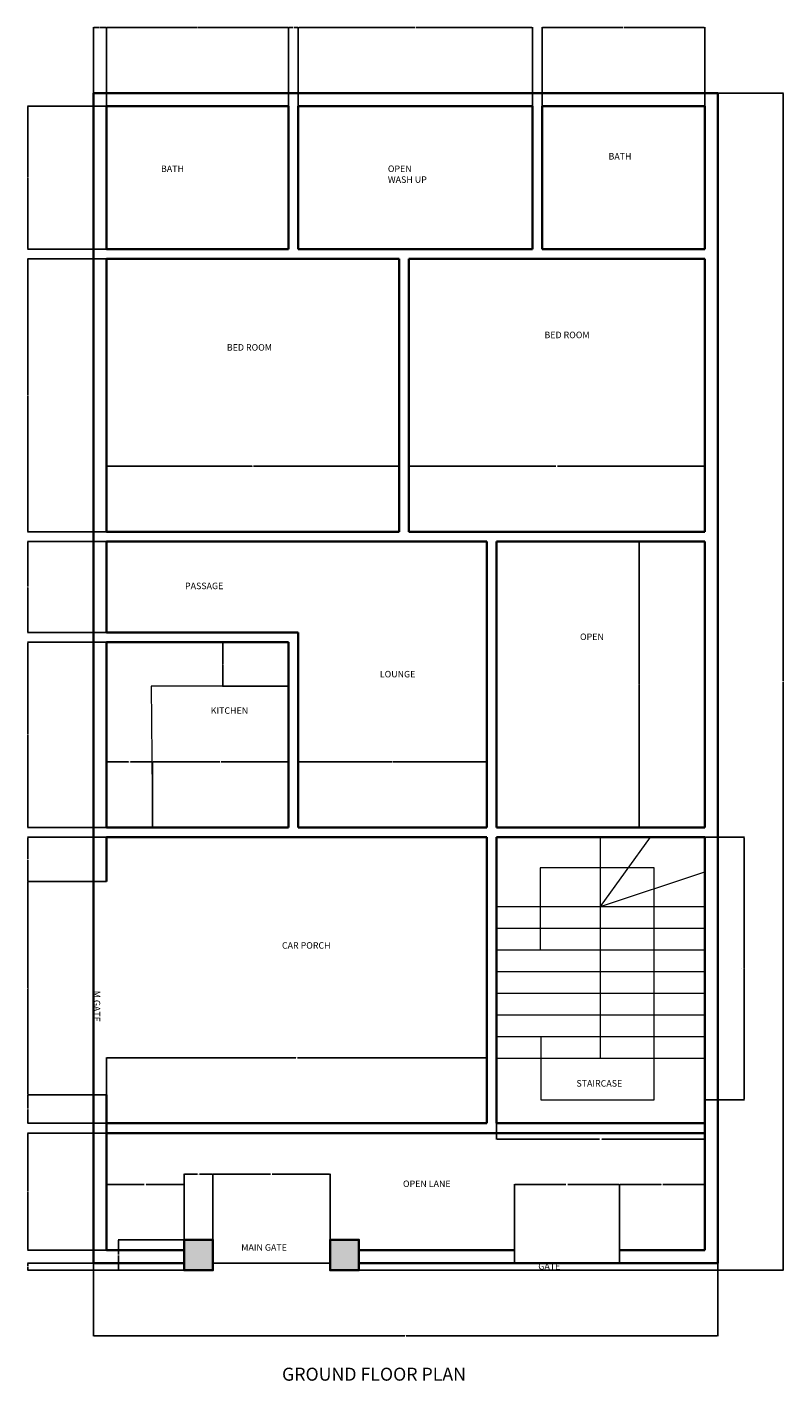
# Model space of a CAD drawing. Units: inches. Extents: x 301 to 1174, y -458 to 167.
# Tile 1 of 4: x 301 to 651, y -458 to 167. Entities that reach past the tile are written whole.
import ezdxf

# ---------------------------------------------------------------- set-up
doc = ezdxf.new("R2010")
doc.units = ezdxf.units.IN
doc.header["$MEASUREMENT"] = 0
for name, color, linetype, lineweight in [('A-ANNO-DIMS', 2, 'Continuous', 18), ('A-ANNO-TEXT', 7, 'Continuous', 25), ('A-AREA-IDEN', 7, 'Continuous', 18), ('A-COLS', 7, 'Continuous', 35), ('A-COLS-PATT', 252, 'Continuous', 13), ('A-DOOR', 3, 'Continuous', 25), ('A-FLOR-FIXT', 8, 'Continuous', 18), ('A-FLOR-STRS', 7, 'Continuous', 18), ('A-WALL', 7, 'Continuous', 35)]:
    doc.layers.add(name, color=color, linetype=linetype, lineweight=lineweight)
doc.styles.get("Standard").update_dxf_attribs({"font": 'arial.ttf'})
doc.dimstyles.get("Standard").update_dxf_attribs({"dimtxt": 0.18, "dimasz": 0.18, "dimexe": 0.18, "dimexo": 0.0625, "dimgap": 0.09, "dimtad": 0, "dimtih": 1, "dimtoh": 1, "dimdec": 4, "dimzin": 0, "dimdsep": 46, "dimtxsty": 'Standard', "dimcen": 0.09, "dimadec": 0, "dimazin": 0, "dimtfac": 1, "dimtdec": 4, "dimtofl": 0, "dimtmove": 0, "dimatfit": 3, "dimfxl": 1, "dimtolj": 1, "dimtzin": 0, "dimarcsym": 0})

# ---------------------------------------------------------------- blocks, each defined once
blk = doc.blocks.new('STAIR-RES-WINDER')
for p, q in [((48, 19.16), (48, 121.12)), ((48, 89.16), (71.07, 121.12)), ((72.66, 107.09), (20.07, 107.09)), ((20.07, 107.09), (20.07, 69.16)), ((72.66, 0), (72.66, 107.09)), ((48, 89.16), (96, 105.1)), ((0, 89.16), (96, 89.16)), ((0, 79.16), (96, 79.16)), ((0, 69.16), (96, 69.16)), ((0, 59.16), (96, 59.16)), ((0, 49.16), (96, 49.16)), ((0, 39.16), (96, 39.16)), ((0, 29.16), (96, 29.16)), ((20.47, 29.16), (20.47, 0)), ((0, 19.16), (96, 19.16)), ((20.47, 0), (72.66, 0))]:
    blk.add_line(p, q)
blk = doc.blocks.new('*D6')
at = {"layer": 'A-ANNO-DIMS', "color": 0, "lineweight": -2, "transparency": 16777216}
for p, q in [((614.09, -206.7), (632.37, -206.7)), ((632.19, -206.88), (632.19, -267.07)), ((632.19, -327.63), (632.19, -267.44)), ((614.09, -327.81), (632.37, -327.81))]:
    blk.add_line(p, q, dxfattribs=at)
at = {"layer": 'A-ANNO-DIMS', "color": 0, "transparency": 16777216}
for points in [[(632.16, -206.88), (632.22, -206.88), (632.19, -206.7)], [(632.16, -327.63), (632.22, -327.63), (632.19, -327.81)]]:
    blk.add_solid(points, dxfattribs=at)
at = {"layer": 'Defpoints', "color": 0, "transparency": 16777216}
for p in [(614.03, -206.7), (632.19, -206.7), (614.03, -327.81)]:
    blk.add_point(p, dxfattribs=at)
at = {"layer": 'A-ANNO-DIMS', "color": 0, "transparency": 16777216, "insert": (632.19, -267.26), "char_height": 0.18, "attachment_point": 5}
blk.add_mtext('\\A1;WINDER STAIR 121 TYP.', dxfattribs=at)
blk = doc.blocks.new('*D7')
at = {"layer": 'A-ANNO-DIMS', "color": 0, "lineweight": -2, "transparency": 16777216}
for p, q in [((518.03, -327.88), (518.03, -346.16)), ((614.03, -327.88), (614.03, -346.16)), ((518.21, -345.98), (565.5, -345.98)), ((613.85, -345.98), (566.55, -345.98))]:
    blk.add_line(p, q, dxfattribs=at)
at = {"layer": 'A-ANNO-DIMS', "color": 0, "transparency": 16777216}
for points in [[(518.21, -345.95), (518.21, -346.01), (518.03, -345.98)], [(613.85, -345.95), (613.85, -346.01), (614.03, -345.98)]]:
    blk.add_solid(points, dxfattribs=at)
at = {"layer": 'Defpoints', "color": 0, "transparency": 16777216}
for p in [(518.03, -327.81), (614.03, -327.81), (614.03, -345.98)]:
    blk.add_point(p, dxfattribs=at)
at = {"layer": 'A-ANNO-DIMS', "color": 0, "transparency": 16777216, "insert": (566.03, -345.98), "char_height": 0.18, "attachment_point": 5}
blk.add_mtext('\\A1;96 TYP.', dxfattribs=at)
blk = doc.blocks.new('*D8')
at = {"layer": 'A-ANNO-DIMS', "color": 0, "lineweight": -2, "transparency": 16777216}
for p, q in [((332.03, -403.26), (332.03, -436.96)), ((620.03, -403.26), (620.03, -436.96)), ((332.21, -436.78), (475.74, -436.78)), ((619.85, -436.78), (476.32, -436.78))]:
    blk.add_line(p, q, dxfattribs=at)
at = {"layer": 'A-ANNO-DIMS', "color": 0, "transparency": 16777216}
for points in [[(332.21, -436.75), (332.21, -436.81), (332.03, -436.78)], [(619.85, -436.75), (619.85, -436.81), (620.03, -436.78)]]:
    blk.add_solid(points, dxfattribs=at)
at = {"layer": 'Defpoints', "color": 0, "transparency": 16777216}
for p in [(332.03, -403.2), (620.03, -403.2), (620.03, -436.78)]:
    blk.add_point(p, dxfattribs=at)
at = {"layer": 'A-ANNO-DIMS', "color": 0, "transparency": 16777216, "insert": (476.03, -436.78), "char_height": 0.18, "attachment_point": 5}
blk.add_mtext('\\A1;288', dxfattribs=at)
blk = doc.blocks.new('*D9')
at = {"layer": 'A-ANNO-DIMS', "color": 0, "lineweight": -2, "transparency": 16777216}
for p, q in [((620.09, 136.8), (650.46, 136.8)), ((650.28, 136.62), (650.28, -134.68)), ((650.28, -406.35), (650.28, -135.05)), ((454.55, -406.53), (650.46, -406.53))]:
    blk.add_line(p, q, dxfattribs=at)
at = {"layer": 'A-ANNO-DIMS', "color": 0, "transparency": 16777216}
for points in [[(650.25, 136.62), (650.31, 136.62), (650.28, 136.8)], [(650.25, -406.35), (650.31, -406.35), (650.28, -406.53)]]:
    blk.add_solid(points, dxfattribs=at)
at = {"layer": 'Defpoints', "color": 0, "transparency": 16777216}
for p in [(620.03, 136.8), (650.28, 136.8), (454.48, -406.53)]:
    blk.add_point(p, dxfattribs=at)
at = {"layer": 'A-ANNO-DIMS', "color": 0, "transparency": 16777216, "insert": (650.28, -134.86), "char_height": 0.18, "attachment_point": 5}
blk.add_mtext('\\A1;543.3', dxfattribs=at)
blk = doc.blocks.new('*D10')
at = {"layer": 'A-ANNO-DIMS', "color": 0, "lineweight": -2, "transparency": 16777216}
for p, q in [((332.03, 136.86), (332.03, 167.23)), ((332.21, 167.05), (334.88, 167.05)), ((337.85, 167.05), (335.17, 167.05)), ((338.03, 130.86), (338.03, 167.23))]:
    blk.add_line(p, q, dxfattribs=at)
at = {"layer": 'A-ANNO-DIMS', "color": 0, "transparency": 16777216}
for points in [[(332.21, 167.08), (332.21, 167.02), (332.03, 167.05)], [(337.85, 167.08), (337.85, 167.02), (338.03, 167.05)]]:
    blk.add_solid(points, dxfattribs=at)
at = {"layer": 'Defpoints', "color": 0, "transparency": 16777216}
for p in [(338.03, 167.05), (332.03, 136.8), (338.03, 130.8)]:
    blk.add_point(p, dxfattribs=at)
at = {"layer": 'A-ANNO-DIMS', "color": 0, "transparency": 16777216, "insert": (335.03, 167.05), "char_height": 0.18, "attachment_point": 5}
blk.add_mtext('\\A1;6', dxfattribs=at)
blk = doc.blocks.new('*D11')
at = {"layer": 'A-ANNO-DIMS', "color": 0, "lineweight": -2, "transparency": 16777216}
for p, q in [((338.03, 130.86), (338.03, 167.23)), ((338.21, 167.05), (379.81, 167.05)), ((421.85, 167.05), (380.24, 167.05)), ((422.03, 130.86), (422.03, 167.23))]:
    blk.add_line(p, q, dxfattribs=at)
at = {"layer": 'A-ANNO-DIMS', "color": 0, "transparency": 16777216}
for points in [[(338.21, 167.08), (338.21, 167.02), (338.03, 167.05)], [(421.85, 167.08), (421.85, 167.02), (422.03, 167.05)]]:
    blk.add_solid(points, dxfattribs=at)
at = {"layer": 'Defpoints', "color": 0, "transparency": 16777216}
for p in [(422.03, 167.05), (338.03, 130.8), (422.03, 130.8)]:
    blk.add_point(p, dxfattribs=at)
at = {"layer": 'A-ANNO-DIMS', "color": 0, "transparency": 16777216, "insert": (380.03, 167.05), "char_height": 0.18, "attachment_point": 5}
blk.add_mtext('\\A1;84', dxfattribs=at)
blk = doc.blocks.new('*D12')
at = {"layer": 'A-ANNO-DIMS', "color": 0, "lineweight": -2, "transparency": 16777216}
for p, q in [((422.03, 130.86), (422.03, 167.23)), ((422.21, 167.05), (424.02, 167.05)), ((426.35, 167.05), (424.53, 167.05)), ((426.53, 130.86), (426.53, 167.23))]:
    blk.add_line(p, q, dxfattribs=at)
at = {"layer": 'A-ANNO-DIMS', "color": 0, "transparency": 16777216}
for points in [[(422.21, 167.08), (422.21, 167.02), (422.03, 167.05)], [(426.35, 167.08), (426.35, 167.02), (426.53, 167.05)]]:
    blk.add_solid(points, dxfattribs=at)
at = {"layer": 'Defpoints', "color": 0, "transparency": 16777216}
for p in [(426.53, 167.05), (422.03, 130.8), (426.53, 130.8)]:
    blk.add_point(p, dxfattribs=at)
at = {"layer": 'A-ANNO-DIMS', "color": 0, "transparency": 16777216, "insert": (424.28, 167.05), "char_height": 0.18, "attachment_point": 5}
blk.add_mtext('\\A1;4.5', dxfattribs=at)
blk = doc.blocks.new('*D13')
at = {"layer": 'A-ANNO-DIMS', "color": 0, "lineweight": -2, "transparency": 16777216}
for p, q in [((426.53, 130.86), (426.53, 167.23)), ((426.71, 167.05), (480.25, 167.05)), ((534.35, 167.05), (480.81, 167.05)), ((534.53, 130.86), (534.53, 167.23))]:
    blk.add_line(p, q, dxfattribs=at)
at = {"layer": 'A-ANNO-DIMS', "color": 0, "transparency": 16777216}
for points in [[(426.71, 167.08), (426.71, 167.02), (426.53, 167.05)], [(534.35, 167.08), (534.35, 167.02), (534.53, 167.05)]]:
    blk.add_solid(points, dxfattribs=at)
at = {"layer": 'Defpoints', "color": 0, "transparency": 16777216}
for p in [(534.53, 167.05), (426.53, 130.8), (534.53, 130.8)]:
    blk.add_point(p, dxfattribs=at)
at = {"layer": 'A-ANNO-DIMS', "color": 0, "transparency": 16777216, "insert": (480.53, 167.05), "char_height": 0.18, "attachment_point": 5}
blk.add_mtext('\\A1;108', dxfattribs=at)
blk = doc.blocks.new('*D14')
at = {"layer": 'A-ANNO-DIMS', "color": 0, "lineweight": -2, "transparency": 16777216}
for p, q in [((539.03, 130.86), (539.03, 167.23)), ((539.21, 167.05), (576.31, 167.05)), ((613.85, 167.05), (576.74, 167.05)), ((614.03, 130.86), (614.03, 167.23))]:
    blk.add_line(p, q, dxfattribs=at)
at = {"layer": 'A-ANNO-DIMS', "color": 0, "transparency": 16777216}
for points in [[(539.21, 167.08), (539.21, 167.02), (539.03, 167.05)], [(613.85, 167.08), (613.85, 167.02), (614.03, 167.05)]]:
    blk.add_solid(points, dxfattribs=at)
at = {"layer": 'Defpoints', "color": 0, "transparency": 16777216}
for p in [(614.03, 167.05), (539.03, 130.8), (614.03, 130.8)]:
    blk.add_point(p, dxfattribs=at)
at = {"layer": 'A-ANNO-DIMS', "color": 0, "transparency": 16777216, "insert": (576.53, 167.05), "char_height": 0.18, "attachment_point": 5}
blk.add_mtext('\\A1;75', dxfattribs=at)
blk = doc.blocks.new('*D15')
at = {"layer": 'A-ANNO-DIMS', "color": 0, "lineweight": -2, "transparency": 16777216}
for p, q in [((338.03, -65.64), (338.03, -35.27)), ((338.21, -35.45), (405.24, -35.45)), ((472.85, -35.45), (405.81, -35.45)), ((473.03, -65.64), (473.03, -35.27))]:
    blk.add_line(p, q, dxfattribs=at)
at = {"layer": 'A-ANNO-DIMS', "color": 0, "transparency": 16777216}
for points in [[(338.21, -35.42), (338.21, -35.48), (338.03, -35.45)], [(472.85, -35.42), (472.85, -35.48), (473.03, -35.45)]]:
    blk.add_solid(points, dxfattribs=at)
at = {"layer": 'Defpoints', "color": 0, "transparency": 16777216}
for p in [(473.03, -35.45), (338.03, -65.7), (473.03, -65.7)]:
    blk.add_point(p, dxfattribs=at)
at = {"layer": 'A-ANNO-DIMS', "color": 0, "transparency": 16777216, "insert": (405.53, -35.45), "char_height": 0.18, "attachment_point": 5}
blk.add_mtext('\\A1;135', dxfattribs=at)
blk = doc.blocks.new('*D16')
at = {"layer": 'A-ANNO-DIMS', "color": 0, "lineweight": -2, "transparency": 16777216}
for p, q in [((477.53, -65.64), (477.53, -35.27)), ((477.71, -35.45), (545.39, -35.45)), ((613.85, -35.45), (546.16, -35.45)), ((614.03, -65.64), (614.03, -35.27))]:
    blk.add_line(p, q, dxfattribs=at)
at = {"layer": 'A-ANNO-DIMS', "color": 0, "transparency": 16777216}
for points in [[(477.71, -35.42), (477.71, -35.48), (477.53, -35.45)], [(613.85, -35.42), (613.85, -35.48), (614.03, -35.45)]]:
    blk.add_solid(points, dxfattribs=at)
at = {"layer": 'Defpoints', "color": 0, "transparency": 16777216}
for p in [(614.03, -35.45), (477.53, -65.7), (614.03, -65.7)]:
    blk.add_point(p, dxfattribs=at)
at = {"layer": 'A-ANNO-DIMS', "color": 0, "transparency": 16777216, "insert": (545.78, -35.45), "char_height": 0.18, "attachment_point": 5}
blk.add_mtext('\\A1;136.5', dxfattribs=at)
blk = doc.blocks.new('*D17')
at = {"layer": 'A-ANNO-DIMS', "color": 0, "lineweight": -2, "transparency": 16777216}
for p, q in [((338.03, -202.14), (338.03, -171.77)), ((338.21, -171.95), (348.21, -171.95)), ((359.15, -171.95), (349.14, -171.95)), ((359.33, -202.14), (359.33, -171.77))]:
    blk.add_line(p, q, dxfattribs=at)
at = {"layer": 'A-ANNO-DIMS', "color": 0, "transparency": 16777216}
for points in [[(338.21, -171.92), (338.21, -171.98), (338.03, -171.95)], [(359.15, -171.92), (359.15, -171.98), (359.33, -171.95)]]:
    blk.add_solid(points, dxfattribs=at)
at = {"layer": 'Defpoints', "color": 0, "transparency": 16777216}
for p in [(359.33, -171.95), (338.03, -202.2), (359.33, -202.2)]:
    blk.add_point(p, dxfattribs=at)
at = {"layer": 'A-ANNO-DIMS', "color": 0, "transparency": 16777216, "insert": (348.68, -171.95), "char_height": 0.18, "attachment_point": 5}
blk.add_mtext('\\A1;21.305', dxfattribs=at)
blk = doc.blocks.new('*D18')
at = {"layer": 'A-ANNO-DIMS', "color": 0, "lineweight": -2, "transparency": 16777216}
for p, q in [((359.33, -202.14), (359.33, -171.77)), ((359.51, -171.95), (390.35, -171.95)), ((421.85, -171.95), (391, -171.95)), ((422.03, -202.14), (422.03, -171.77))]:
    blk.add_line(p, q, dxfattribs=at)
at = {"layer": 'A-ANNO-DIMS', "color": 0, "transparency": 16777216}
for points in [[(359.51, -171.92), (359.51, -171.98), (359.33, -171.95)], [(421.85, -171.92), (421.85, -171.98), (422.03, -171.95)]]:
    blk.add_solid(points, dxfattribs=at)
at = {"layer": 'Defpoints', "color": 0, "transparency": 16777216}
for p in [(422.03, -171.95), (359.33, -202.2), (422.03, -202.2)]:
    blk.add_point(p, dxfattribs=at)
at = {"layer": 'A-ANNO-DIMS', "color": 0, "transparency": 16777216, "insert": (390.68, -171.95), "char_height": 0.18, "attachment_point": 5}
blk.add_mtext('\\A1;62.7', dxfattribs=at)
blk = doc.blocks.new('*D19')
at = {"layer": 'A-ANNO-DIMS', "color": 0, "lineweight": -2, "transparency": 16777216}
for p, q in [((426.53, -202.14), (426.53, -171.77)), ((426.71, -171.95), (469.81, -171.95)), ((513.35, -171.95), (470.24, -171.95)), ((513.53, -202.14), (513.53, -171.77))]:
    blk.add_line(p, q, dxfattribs=at)
at = {"layer": 'A-ANNO-DIMS', "color": 0, "transparency": 16777216}
for points in [[(426.71, -171.92), (426.71, -171.98), (426.53, -171.95)], [(513.35, -171.92), (513.35, -171.98), (513.53, -171.95)]]:
    blk.add_solid(points, dxfattribs=at)
at = {"layer": 'Defpoints', "color": 0, "transparency": 16777216}
for p in [(513.53, -171.95), (426.53, -202.2), (513.53, -202.2)]:
    blk.add_point(p, dxfattribs=at)
at = {"layer": 'A-ANNO-DIMS', "color": 0, "transparency": 16777216, "insert": (470.03, -171.95), "char_height": 0.18, "attachment_point": 5}
blk.add_mtext('\\A1;87', dxfattribs=at)
blk = doc.blocks.new('*D20')
at = {"layer": 'A-ANNO-DIMS', "color": 0, "lineweight": -2, "transparency": 16777216}
for p, q in [((338.03, -338.64), (338.03, -308.27)), ((338.21, -308.45), (425.39, -308.45)), ((513.35, -308.45), (426.16, -308.45)), ((513.53, -338.64), (513.53, -308.27))]:
    blk.add_line(p, q, dxfattribs=at)
at = {"layer": 'A-ANNO-DIMS', "color": 0, "transparency": 16777216}
for points in [[(338.21, -308.42), (338.21, -308.48), (338.03, -308.45)], [(513.35, -308.42), (513.35, -308.48), (513.53, -308.45)]]:
    blk.add_solid(points, dxfattribs=at)
at = {"layer": 'Defpoints', "color": 0, "transparency": 16777216}
for p in [(513.53, -308.45), (338.03, -338.7), (513.53, -338.7)]:
    blk.add_point(p, dxfattribs=at)
at = {"layer": 'A-ANNO-DIMS', "color": 0, "transparency": 16777216, "insert": (425.78, -308.45), "char_height": 0.18, "attachment_point": 5}
blk.add_mtext('\\A1;175.5', dxfattribs=at)
blk = doc.blocks.new('*D21')
at = {"layer": 'A-ANNO-DIMS', "color": 0, "lineweight": -2, "transparency": 16777216}
for p, q in [((337.96, 130.8), (301.6, 130.8)), ((301.78, 130.62), (301.78, 97.98)), ((301.78, 64.98), (301.78, 97.62)), ((337.96, 64.8), (301.6, 64.8))]:
    blk.add_line(p, q, dxfattribs=at)
at = {"layer": 'A-ANNO-DIMS', "color": 0, "transparency": 16777216}
for points in [[(301.75, 130.62), (301.81, 130.62), (301.78, 130.8)], [(301.75, 64.98), (301.81, 64.98), (301.78, 64.8)]]:
    blk.add_solid(points, dxfattribs=at)
at = {"layer": 'Defpoints', "color": 0, "transparency": 16777216}
for p in [(301.78, 130.8), (338.03, 130.8), (338.03, 64.8)]:
    blk.add_point(p, dxfattribs=at)
at = {"layer": 'A-ANNO-DIMS', "color": 0, "transparency": 16777216, "insert": (301.78, 97.8), "char_height": 0.18, "attachment_point": 5}
blk.add_mtext('\\A1;66', dxfattribs=at)
blk = doc.blocks.new('*D22')
at = {"layer": 'A-ANNO-DIMS', "color": 0, "lineweight": -2, "transparency": 16777216}
for p, q in [((337.96, 60.3), (301.6, 60.3)), ((301.78, 60.12), (301.78, -2.52)), ((301.78, -65.52), (301.78, -2.88)), ((337.96, -65.7), (301.6, -65.7))]:
    blk.add_line(p, q, dxfattribs=at)
at = {"layer": 'A-ANNO-DIMS', "color": 0, "transparency": 16777216}
for points in [[(301.75, 60.12), (301.81, 60.12), (301.78, 60.3)], [(301.75, -65.52), (301.81, -65.52), (301.78, -65.7)]]:
    blk.add_solid(points, dxfattribs=at)
at = {"layer": 'Defpoints', "color": 0, "transparency": 16777216}
for p in [(301.78, 60.3), (338.03, 60.3), (338.03, -65.7)]:
    blk.add_point(p, dxfattribs=at)
at = {"layer": 'A-ANNO-DIMS', "color": 0, "transparency": 16777216, "insert": (301.78, -2.7), "char_height": 0.18, "attachment_point": 5}
blk.add_mtext('\\A1;126', dxfattribs=at)
blk = doc.blocks.new('*D23')
at = {"layer": 'A-ANNO-DIMS', "color": 0, "lineweight": -2, "transparency": 16777216}
for p, q in [((337.96, -70.2), (301.6, -70.2)), ((301.78, -70.38), (301.78, -91.02)), ((301.78, -112.02), (301.78, -91.38)), ((337.96, -112.2), (301.6, -112.2))]:
    blk.add_line(p, q, dxfattribs=at)
at = {"layer": 'A-ANNO-DIMS', "color": 0, "transparency": 16777216}
for points in [[(301.75, -70.38), (301.81, -70.38), (301.78, -70.2)], [(301.75, -112.02), (301.81, -112.02), (301.78, -112.2)]]:
    blk.add_solid(points, dxfattribs=at)
at = {"layer": 'Defpoints', "color": 0, "transparency": 16777216}
for p in [(301.78, -70.2), (338.03, -70.2), (338.03, -112.2)]:
    blk.add_point(p, dxfattribs=at)
at = {"layer": 'A-ANNO-DIMS', "color": 0, "transparency": 16777216, "insert": (301.78, -91.2), "char_height": 0.18, "attachment_point": 5}
blk.add_mtext('\\A1;42', dxfattribs=at)
blk = doc.blocks.new('*D24')
at = {"layer": 'A-ANNO-DIMS', "color": 0, "lineweight": -2, "transparency": 16777216}
for p, q in [((337.96, -116.7), (301.6, -116.7)), ((301.78, -116.88), (301.78, -159.27)), ((301.78, -202.02), (301.78, -159.63)), ((337.96, -202.2), (301.6, -202.2))]:
    blk.add_line(p, q, dxfattribs=at)
at = {"layer": 'A-ANNO-DIMS', "color": 0, "transparency": 16777216}
for points in [[(301.75, -116.88), (301.81, -116.88), (301.78, -116.7)], [(301.75, -202.02), (301.81, -202.02), (301.78, -202.2)]]:
    blk.add_solid(points, dxfattribs=at)
at = {"layer": 'Defpoints', "color": 0, "transparency": 16777216}
for p in [(301.78, -116.7), (338.03, -116.7), (338.03, -202.2)]:
    blk.add_point(p, dxfattribs=at)
at = {"layer": 'A-ANNO-DIMS', "color": 0, "transparency": 16777216, "insert": (301.78, -159.45), "char_height": 0.18, "attachment_point": 5}
blk.add_mtext('\\A1;85.5', dxfattribs=at)
blk = doc.blocks.new('*D25')
at = {"layer": 'A-ANNO-DIMS', "color": 0, "lineweight": -2, "transparency": 16777216}
for p, q in [((337.96, -325.51), (301.6, -325.51)), ((301.78, -325.69), (301.78, -331.92)), ((301.78, -338.52), (301.78, -332.29)), ((337.96, -338.7), (301.6, -338.7))]:
    blk.add_line(p, q, dxfattribs=at)
at = {"layer": 'A-ANNO-DIMS', "color": 0, "transparency": 16777216}
for points in [[(301.75, -325.69), (301.81, -325.69), (301.78, -325.51)], [(301.75, -338.52), (301.81, -338.52), (301.78, -338.7)]]:
    blk.add_solid(points, dxfattribs=at)
at = {"layer": 'Defpoints', "color": 0, "transparency": 16777216}
for p in [(301.78, -325.51), (338.03, -325.51), (338.03, -338.7)]:
    blk.add_point(p, dxfattribs=at)
at = {"layer": 'A-ANNO-DIMS', "color": 0, "transparency": 16777216, "insert": (301.78, -332.1), "char_height": 0.18, "attachment_point": 5}
blk.add_mtext('\\A1;13.19', dxfattribs=at)
blk = doc.blocks.new('*D26')
at = {"layer": 'A-ANNO-DIMS', "color": 0, "lineweight": -2, "transparency": 16777216}
for p, q in [((337.96, -227.07), (301.6, -227.07)), ((301.78, -227.25), (301.78, -276.11)), ((301.78, -325.33), (301.78, -276.47)), ((337.96, -325.51), (301.6, -325.51))]:
    blk.add_line(p, q, dxfattribs=at)
at = {"layer": 'A-ANNO-DIMS', "color": 0, "transparency": 16777216}
for points in [[(301.75, -227.25), (301.81, -227.25), (301.78, -227.07)], [(301.75, -325.33), (301.81, -325.33), (301.78, -325.51)]]:
    blk.add_solid(points, dxfattribs=at)
at = {"layer": 'Defpoints', "color": 0, "transparency": 16777216}
for p in [(301.78, -227.07), (338.03, -227.07), (338.03, -325.51)]:
    blk.add_point(p, dxfattribs=at)
at = {"layer": 'A-ANNO-DIMS', "color": 0, "transparency": 16777216, "insert": (301.78, -276.29), "char_height": 0.18, "attachment_point": 5}
blk.add_mtext('\\A1;98.44', dxfattribs=at)
blk = doc.blocks.new('*D27')
at = {"layer": 'A-ANNO-DIMS', "color": 0, "lineweight": -2, "transparency": 16777216}
for p, q in [((337.96, -206.7), (301.6, -206.7)), ((301.78, -206.88), (301.78, -216.7)), ((301.78, -226.89), (301.78, -217.07)), ((337.96, -227.07), (301.6, -227.07))]:
    blk.add_line(p, q, dxfattribs=at)
at = {"layer": 'A-ANNO-DIMS', "color": 0, "transparency": 16777216}
for points in [[(301.75, -206.88), (301.81, -206.88), (301.78, -206.7)], [(301.75, -226.89), (301.81, -226.89), (301.78, -227.07)]]:
    blk.add_solid(points, dxfattribs=at)
at = {"layer": 'Defpoints', "color": 0, "transparency": 16777216}
for p in [(301.78, -206.7), (338.03, -206.7), (338.03, -227.07)]:
    blk.add_point(p, dxfattribs=at)
at = {"layer": 'A-ANNO-DIMS', "color": 0, "transparency": 16777216, "insert": (301.78, -216.89), "char_height": 0.18, "attachment_point": 5}
blk.add_mtext('\\A1;20.375', dxfattribs=at)
blk = doc.blocks.new('*D28')
at = {"layer": 'A-ANNO-DIMS', "color": 0, "lineweight": -2, "transparency": 16777216}
for p, q in [((337.96, -343.2), (301.6, -343.2)), ((301.78, -343.38), (301.78, -370.02)), ((301.78, -397.02), (301.78, -370.38)), ((337.96, -397.2), (301.6, -397.2))]:
    blk.add_line(p, q, dxfattribs=at)
at = {"layer": 'A-ANNO-DIMS', "color": 0, "transparency": 16777216}
for points in [[(301.75, -343.38), (301.81, -343.38), (301.78, -343.2)], [(301.75, -397.02), (301.81, -397.02), (301.78, -397.2)]]:
    blk.add_solid(points, dxfattribs=at)
at = {"layer": 'Defpoints', "color": 0, "transparency": 16777216}
for p in [(301.78, -343.2), (338.03, -343.2), (338.03, -397.2)]:
    blk.add_point(p, dxfattribs=at)
at = {"layer": 'A-ANNO-DIMS', "color": 0, "transparency": 16777216, "insert": (301.78, -370.2), "char_height": 0.18, "attachment_point": 5}
blk.add_mtext('\\A1;54', dxfattribs=at)
blk = doc.blocks.new('*D29')
at = {"layer": 'A-ANNO-DIMS', "color": 0, "lineweight": -2, "transparency": 16777216}
for p, q in [((338.03, -397.14), (338.03, -366.77)), ((338.21, -366.95), (355.45, -366.95)), ((373.63, -366.95), (356.38, -366.95)), ((373.81, -397.14), (373.81, -366.77))]:
    blk.add_line(p, q, dxfattribs=at)
at = {"layer": 'A-ANNO-DIMS', "color": 0, "transparency": 16777216}
for points in [[(338.21, -366.92), (338.21, -366.98), (338.03, -366.95)], [(373.63, -366.92), (373.63, -366.98), (373.81, -366.95)]]:
    blk.add_solid(points, dxfattribs=at)
at = {"layer": 'Defpoints', "color": 0, "transparency": 16777216}
for p in [(373.81, -366.95), (338.03, -397.2), (373.81, -397.2)]:
    blk.add_point(p, dxfattribs=at)
at = {"layer": 'A-ANNO-DIMS', "color": 0, "transparency": 16777216, "insert": (355.92, -366.95), "char_height": 0.18, "attachment_point": 5}
blk.add_mtext('\\A1;35.785', dxfattribs=at)
blk = doc.blocks.new('*D30')
at = {"layer": 'A-ANNO-DIMS', "color": 0, "lineweight": -2, "transparency": 16777216}
for p, q in [((387.13, -392.41), (387.13, -362.04)), ((387.31, -362.22), (413.75, -362.22)), ((440.99, -362.22), (414.54, -362.22)), ((441.17, -392.41), (441.17, -362.04))]:
    blk.add_line(p, q, dxfattribs=at)
at = {"layer": 'A-ANNO-DIMS', "color": 0, "transparency": 16777216}
for points in [[(387.31, -362.19), (387.31, -362.25), (387.13, -362.22)], [(440.99, -362.19), (440.99, -362.25), (441.17, -362.22)]]:
    blk.add_solid(points, dxfattribs=at)
at = {"layer": 'Defpoints', "color": 0, "transparency": 16777216}
for p in [(441.17, -362.22), (387.13, -392.47), (441.17, -392.47)]:
    blk.add_point(p, dxfattribs=at)
at = {"layer": 'A-ANNO-DIMS', "color": 0, "transparency": 16777216, "insert": (414.15, -362.22), "char_height": 0.18, "attachment_point": 5}
blk.add_mtext('\\A1;54.04', dxfattribs=at)
blk = doc.blocks.new('*D31')
at = {"layer": 'A-ANNO-DIMS', "color": 0, "lineweight": -2, "transparency": 16777216}
for p, q in [((373.81, -392.41), (373.81, -362.04)), ((373.99, -362.22), (380.01, -362.22)), ((386.95, -362.22), (380.93, -362.22)), ((387.13, -392.41), (387.13, -362.04))]:
    blk.add_line(p, q, dxfattribs=at)
at = {"layer": 'A-ANNO-DIMS', "color": 0, "transparency": 16777216}
for points in [[(373.99, -362.19), (373.99, -362.25), (373.81, -362.22)], [(386.95, -362.19), (386.95, -362.25), (387.13, -362.22)]]:
    blk.add_solid(points, dxfattribs=at)
at = {"layer": 'Defpoints', "color": 0, "transparency": 16777216}
for p in [(387.13, -362.22), (373.81, -392.47), (387.13, -392.47)]:
    blk.add_point(p, dxfattribs=at)
at = {"layer": 'A-ANNO-DIMS', "color": 0, "transparency": 16777216, "insert": (380.47, -362.22), "char_height": 0.18, "attachment_point": 5}
blk.add_mtext('\\A1;13.318', dxfattribs=at)
blk = doc.blocks.new('*D32')
at = {"layer": 'A-ANNO-DIMS', "color": 0, "lineweight": -2, "transparency": 16777216}
for p, q in [((373.75, -392.47), (343.38, -392.47)), ((343.56, -392.65), (343.56, -399.32)), ((343.56, -406.35), (343.56, -399.68)), ((373.75, -406.53), (343.38, -406.53))]:
    blk.add_line(p, q, dxfattribs=at)
at = {"layer": 'A-ANNO-DIMS', "color": 0, "transparency": 16777216}
for points in [[(343.53, -392.65), (343.59, -392.65), (343.56, -392.47)], [(343.53, -406.35), (343.59, -406.35), (343.56, -406.53)]]:
    blk.add_solid(points, dxfattribs=at)
at = {"layer": 'Defpoints', "color": 0, "transparency": 16777216}
for p in [(343.56, -392.47), (373.81, -392.47), (373.81, -406.53)]:
    blk.add_point(p, dxfattribs=at)
at = {"layer": 'A-ANNO-DIMS', "color": 0, "transparency": 16777216, "insert": (343.56, -399.5), "char_height": 0.18, "attachment_point": 5}
blk.add_mtext('\\A1;14.06', dxfattribs=at)
blk = doc.blocks.new('*D33')
at = {"layer": 'A-ANNO-DIMS', "color": 0, "lineweight": -2, "transparency": 16777216}
for p, q in [((331.96, -403.2), (301.6, -403.2)), ((301.78, -403.38), (301.78, -404.68)), ((301.78, -406.35), (301.78, -405.05)), ((373.75, -406.53), (301.6, -406.53))]:
    blk.add_line(p, q, dxfattribs=at)
at = {"layer": 'A-ANNO-DIMS', "color": 0, "transparency": 16777216}
for points in [[(301.75, -403.38), (301.81, -403.38), (301.78, -403.2)], [(301.75, -406.35), (301.81, -406.35), (301.78, -406.53)]]:
    blk.add_solid(points, dxfattribs=at)
at = {"layer": 'Defpoints', "color": 0, "transparency": 16777216}
for p in [(301.78, -403.2), (332.03, -403.2), (373.81, -406.53)]:
    blk.add_point(p, dxfattribs=at)
at = {"layer": 'A-ANNO-DIMS', "color": 0, "transparency": 16777216, "insert": (301.78, -404.86), "char_height": 0.18, "attachment_point": 5}
blk.add_mtext('\\A1;3.33', dxfattribs=at)
blk = doc.blocks.new('*D34')
at = {"layer": 'A-ANNO-DIMS', "color": 0, "lineweight": -2, "transparency": 16777216}
for p, q in [((526.22, -397.14), (526.22, -366.77)), ((526.4, -366.95), (550.04, -366.95)), ((574.47, -366.95), (550.83, -366.95)), ((574.65, -397.14), (574.65, -366.77))]:
    blk.add_line(p, q, dxfattribs=at)
at = {"layer": 'A-ANNO-DIMS', "color": 0, "transparency": 16777216}
for points in [[(526.4, -366.92), (526.4, -366.98), (526.22, -366.95)], [(574.47, -366.92), (574.47, -366.98), (574.65, -366.95)]]:
    blk.add_solid(points, dxfattribs=at)
at = {"layer": 'Defpoints', "color": 0, "transparency": 16777216}
for p in [(574.65, -366.95), (526.22, -397.2), (574.65, -397.2)]:
    blk.add_point(p, dxfattribs=at)
at = {"layer": 'A-ANNO-DIMS', "color": 0, "transparency": 16777216, "insert": (550.44, -366.95), "char_height": 0.18, "attachment_point": 5}
blk.add_mtext('\\A1;48.43', dxfattribs=at)
blk = doc.blocks.new('*D35')
at = {"layer": 'A-ANNO-DIMS', "color": 0, "lineweight": -2, "transparency": 16777216}
for p, q in [((574.65, -397.14), (574.65, -366.77)), ((574.83, -366.95), (593.95, -366.95)), ((613.85, -366.95), (594.73, -366.95)), ((614.03, -397.14), (614.03, -366.77))]:
    blk.add_line(p, q, dxfattribs=at)
at = {"layer": 'A-ANNO-DIMS', "color": 0, "transparency": 16777216}
for points in [[(574.83, -366.92), (574.83, -366.98), (574.65, -366.95)], [(613.85, -366.92), (613.85, -366.98), (614.03, -366.95)]]:
    blk.add_solid(points, dxfattribs=at)
at = {"layer": 'Defpoints', "color": 0, "transparency": 16777216}
for p in [(614.03, -366.95), (574.65, -397.2), (614.03, -397.2)]:
    blk.add_point(p, dxfattribs=at)
at = {"layer": 'A-ANNO-DIMS', "color": 0, "transparency": 16777216, "insert": (594.34, -366.95), "char_height": 0.18, "attachment_point": 5}
blk.add_mtext('\\A1;39.37', dxfattribs=at)
blk = doc.blocks.new('*D36')
at = {"layer": 'A-ANNO-DIMS', "color": 0, "lineweight": -2, "transparency": 16777216}
for p, q in [((421.96, -116.7), (391.6, -116.7)), ((391.78, -116.88), (391.78, -126.64)), ((391.78, -136.76), (391.78, -127)), ((421.96, -136.94), (391.6, -136.94))]:
    blk.add_line(p, q, dxfattribs=at)
at = {"layer": 'A-ANNO-DIMS', "color": 0, "transparency": 16777216}
for points in [[(391.75, -116.88), (391.81, -116.88), (391.78, -116.7)], [(391.75, -136.76), (391.81, -136.76), (391.78, -136.94)]]:
    blk.add_solid(points, dxfattribs=at)
at = {"layer": 'Defpoints', "color": 0, "transparency": 16777216}
for p in [(391.78, -116.7), (422.03, -116.7), (422.03, -136.94)]:
    blk.add_point(p, dxfattribs=at)
at = {"layer": 'A-ANNO-DIMS', "color": 0, "transparency": 16777216, "insert": (391.78, -126.82), "char_height": 0.18, "attachment_point": 5}
blk.add_mtext('\\A1;20.24', dxfattribs=at)
blk = doc.blocks.new('*D37')
at = {"layer": 'A-ANNO-DIMS', "color": 0, "lineweight": -2, "transparency": 16777216}
for p, q in [((613.96, -70.2), (583.6, -70.2)), ((583.78, -70.38), (583.78, -136.02)), ((583.78, -202.02), (583.78, -136.38)), ((613.96, -202.2), (583.6, -202.2))]:
    blk.add_line(p, q, dxfattribs=at)
at = {"layer": 'A-ANNO-DIMS', "color": 0, "transparency": 16777216}
for points in [[(583.75, -70.38), (583.81, -70.38), (583.78, -70.2)], [(583.75, -202.02), (583.81, -202.02), (583.78, -202.2)]]:
    blk.add_solid(points, dxfattribs=at)
at = {"layer": 'Defpoints', "color": 0, "transparency": 16777216}
for p in [(583.78, -70.2), (614.03, -70.2), (614.03, -202.2)]:
    blk.add_point(p, dxfattribs=at)
at = {"layer": 'A-ANNO-DIMS', "color": 0, "transparency": 16777216, "insert": (583.78, -136.2), "char_height": 0.18, "attachment_point": 5}
blk.add_mtext('\\A1;132', dxfattribs=at)

msp = doc.modelspace()

# ---------------------------------------------------------------- hatches: boundary and pattern name
at = {"layer": 'A-COLS-PATT'}
h = msp.add_hatch(color=256, dxfattribs=at)
h.dxf.hatch_style = 1
h.paths.add_polyline_path([(387.1288, -392.4681), (373.8107, -392.4681), (373.8107, -397.1987), (373.8107, -403.1987), (373.8107, -406.5288), (387.1288, -406.5288)])
h.paths.add_polyline_path([(454.4844, -392.4681), (441.1663, -392.4681), (441.1663, -397.1987), (441.1663, -403.1987), (441.1663, -406.5288), (454.4844, -406.5288)])

# ---------------------------------------------------------------- linework, layer by layer
at = {"layer": 'A-COLS'}
for points in [[(373.8107, -403.1987), (373.8107, -397.1987), (373.8107, -392.4681), (387.1288, -392.4681), (387.1288, -406.5288), (373.8107, -406.5288)], [(441.1663, -403.1987), (441.1663, -397.1987), (441.1663, -392.4681), (454.4844, -392.4681), (454.4844, -406.5288), (441.1663, -406.5288)]]:
    msp.add_lwpolyline(points, close=True, dxfattribs=at)
at = {"layer": 'A-DOOR'}
for p, q in [((332.0256, -227.0735), (338.0256, -227.0735)), ((332.0256, -325.5088), (338.0256, -325.5088)), ((526.2185, -397.1987), (526.2185, -403.1987)), ((574.6522, -397.1987), (574.6522, -403.1987)), ((441.1663, -403.1987), (387.1288, -403.1987))]:
    msp.add_line(p, q, dxfattribs=at)
at = {"layer": 'A-FLOR-FIXT'}
for p, q in [((422.0256, -136.9404), (358.7222, -136.9404)), ((358.7222, -136.9404), (359.3302, -202.1987))]:
    msp.add_line(p, q, dxfattribs=at)
at = {"layer": 'A-WALL'}
for p, q in [((332.0256, 136.8013), (620.0256, 136.8013)), ((332.0256, -403.1987), (332.0256, 136.8013)), ((620.0256, 136.8013), (620.0256, -403.1987)), ((338.0256, 130.8013), (422.0256, 130.8013)), ((338.0256, 64.8013), (338.0256, 130.8013)), ((422.0256, 130.8013), (422.0256, 64.8013)), ((426.5256, 130.8013), (426.5256, 64.8013)), ((426.5256, 130.8013), (534.5256, 130.8013)), ((534.5256, 64.8013), (534.5256, 130.8013)), ((539.0256, 64.8013), (539.0256, 130.8013)), ((539.0256, 130.8013), (614.0256, 130.8013)), ((614.0256, 130.8013), (614.0256, 64.8013)), ((422.0256, 64.8013), (338.0256, 64.8013)), ((426.5256, 64.8013), (534.5256, 64.8013)), ((539.0256, 64.8013), (614.0256, 64.8013)), ((422.0256, 60.3013), (338.0256, 60.3013)), ((338.0256, 60.3013), (338.0256, -65.6987)), ((338.0256, -65.6987), (338.0256, 60.3013)), ((422.0256, 60.3013), (426.5256, 60.3013)), ((426.5256, 60.3013), (473.0256, 60.3013)), ((473.0256, -65.6987), (473.0256, 60.3013)), ((477.5256, -65.6987), (477.5256, 60.3013)), ((477.5256, 60.3013), (534.5256, 60.3013)), ((534.5256, 60.3013), (539.0546, 60.3013)), ((539.0256, 60.3013), (614.0256, 60.3013)), ((614.0256, 60.3013), (614.0256, -65.6987)), ((338.0256, -65.6987), (473.0256, -65.6987)), ((477.5256, -65.6987), (614.0256, -65.6987)), ((338.0256, -70.1987), (473.0256, -70.1987)), ((338.0256, -112.1987), (338.0256, -70.1987)), ((473.0256, -70.1987), (513.5256, -70.1987)), ((513.5256, -70.1987), (513.5256, -202.1987)), ((518.0256, -70.1987), (518.0256, -202.1987)), ((518.0256, -70.1987), (614.0256, -70.1987)), ((614.0256, -70.1987), (614.0256, -202.1987)), ((338.0256, -112.1987), (422.0256, -112.1987)), ((422.0256, -112.1987), (426.5256, -112.1987)), ((426.5256, -112.1987), (426.5256, -202.1987)), ((338.0256, -116.6987), (422.0256, -116.6987)), ((338.0256, -202.1987), (338.0256, -116.6987)), ((422.0256, -116.6987), (422.0256, -202.1987)), ((422.0256, -202.1987), (338.0256, -202.1987)), ((426.5256, -202.1987), (513.5256, -202.1987)), ((518.0256, -202.1987), (614.0256, -202.1987)), ((422.0256, -206.6987), (338.0256, -206.6987)), ((338.0256, -227.0735), (338.0256, -206.6987)), ((422.0256, -206.6987), (513.5256, -206.6987)), ((513.5256, -206.6987), (513.5256, -338.6987)), ((518.0256, -206.6987), (518.0256, -338.6987)), ((518.0256, -206.6987), (614.0256, -206.6987)), ((614.0256, -206.6987), (614.0256, -397.1987)), ((338.0256, -397.1987), (338.0256, -325.5088)), ((338.0256, -338.6987), (513.5256, -338.6987)), ((338.0256, -343.1987), (614.0256, -343.1987)), ((518.0256, -338.6987), (614.0256, -338.6987)), ((373.8107, -397.1987), (338.0256, -397.1987)), ((454.4844, -397.1987), (454.4844, -403.1987)), ((526.2185, -397.1987), (454.4844, -397.1987)), ((614.0256, -397.1987), (574.6522, -397.1987)), ((373.8107, -403.1987), (332.0256, -403.1987)), ((620.0256, -403.1987), (454.4844, -403.1987))]:
    msp.add_line(p, q, dxfattribs=at)

# ---------------------------------------------------------------- block references
at = {"layer": 'A-FLOR-STRS'}
msp.add_blockref('STAIR-RES-WINDER', (518.0256, -327.8143), dxfattribs=at)

# ---------------------------------------------------------------- texts
at = {"layer": 'A-ANNO-TEXT', "insert": (335.1299, -277.4892), "char_height": 0.2, "attachment_point": 1, "rotation": 270}
msp.add_mtext_dynamic_manual_height_columns('{\\H15x;M GATE}', width=70.987625, gutter_width=1, heights=[0], dxfattribs=at)
at = {"layer": 'A-ANNO-TEXT', "attachment_point": 1}
for s, width, insert, char_height in [('{\\H15x;MAIN GATE}', 70.987625, (400.2154, -394.4876), 0.2), ('{\\H15x;GATE}', 70.987625, (537.255, -403.1987), 0.2), ('GROUND FLOOR PLAN', 138.96688, (419.0384, -451.4928), 6)]:
    msp.add_mtext_dynamic_manual_height_columns(s, width=width, gutter_width=1, heights=[0], dxfattribs=dict(at, insert=insert, char_height=char_height))
at = {"layer": 'A-AREA-IDEN', "char_height": 0.2, "attachment_point": 1}
for s, insert in [('{\\H15x;BATH}', (569.6586, 109.0828)), ('{\\H15x;BATH}', (363.1808, 103.3405)), ('{\\H15x;OPEN \\PWASH UP}', (467.8564, 103.3405)), ('{\\H15x;BED ROOM}', (540.1031, 26.6399)), ('{\\H15x;BED ROOM}', (393.5572, 20.8976)), ('{\\H15x;PASSAGE}', (374.2641, -89.1891)), ('{\\H15x;OPEN}', (556.5074, -112.6785)), ('{\\H15x;LOUNGE}', (464.1466, -129.9054)), ('{\\H15x;KITCHEN}', (386.153, -146.7221)), ('{\\H15x;CAR PORCH}', (418.9879, -255.1128)), ('{\\H15x;STAIRCASE}', (554.8646, -318.7701)), ('{\\H15x;OPEN LANE}', (474.8185, -365.1186))]:
    msp.add_mtext_dynamic_manual_height_columns(s, width=70.987625, gutter_width=1, heights=[0], dxfattribs=dict(at, insert=insert))

# ---------------------------------------------------------------- dimensions: what is measured, and where the dimension line sits
at = {"layer": 'A-ANNO-DIMS'}
for base, p1, p2, override, picture, middle in [((338.0256, 167.0513), (332.0256, 136.8013), (338.0256, 130.8013), {"dimdec": 0, "dimlfac": 1, "dimrnd": 0, "dimzin": 0, "dimdsep": 46, "dimlunit": 2}, '*D10', (335.0256, 167.0513)), ((422.0256, 167.0513), (338.0256, 130.8013), (422.0256, 130.8013), {"dimdec": 0, "dimlfac": 1, "dimrnd": 0, "dimzin": 0, "dimdsep": 46, "dimlunit": 2}, '*D11', (380.0256, 167.0513)), ((426.5256, 167.0513), (422.0256, 130.8013), (426.5256, 130.8013), {"dimdec": 1, "dimlfac": 1, "dimrnd": 0, "dimzin": 0, "dimdsep": 46, "dimlunit": 2}, '*D12', (424.2756, 167.0513)), ((534.5256, 167.0513), (426.5256, 130.8013), (534.5256, 130.8013), {"dimdec": 0, "dimlfac": 1, "dimrnd": 0, "dimzin": 0, "dimdsep": 46, "dimlunit": 2}, '*D13', (480.5256, 167.0513)), ((614.0256, 167.0513), (539.0256, 130.8013), (614.0256, 130.8013), {"dimdec": 0, "dimlfac": 1, "dimrnd": 0, "dimzin": 0, "dimdsep": 46, "dimlunit": 2}, '*D14', (576.5256, 167.0513)), ((473.0256, -35.4487), (338.0256, -65.6987), (473.0256, -65.6987), {"dimdec": 0, "dimlfac": 1, "dimrnd": 0, "dimzin": 0, "dimdsep": 46, "dimlunit": 2}, '*D15', (405.5256, -35.4487)), ((359.3302, -171.9487), (338.0256, -202.1987), (359.3302, -202.1987), {"dimdec": 3, "dimlfac": 1, "dimrnd": 0, "dimzin": 0, "dimdsep": 46, "dimlunit": 2}, '*D17', (348.6779, -171.9487)), ((513.5256, -308.4487), (338.0256, -338.6987), (513.5256, -338.6987), {"dimdec": 1, "dimlfac": 1, "dimrnd": 0, "dimzin": 0, "dimdsep": 46, "dimlunit": 2}, '*D20', (425.7756, -308.4487)), ((387.1288, -362.2181), (373.8107, -392.4681), (387.1288, -392.4681), {"dimdec": 3, "dimlfac": 1, "dimrnd": 0, "dimzin": 0, "dimdsep": 46, "dimlunit": 2}, '*D31', (380.4698, -362.2181)), ((441.1663, -362.2181), (387.1288, -392.4681), (441.1663, -392.4681), {"dimdec": 2, "dimlfac": 1, "dimrnd": 0, "dimzin": 0, "dimdsep": 46, "dimlunit": 2}, '*D30', (414.1475, -362.2181)), ((373.8107, -366.9487), (338.0256, -397.1987), (373.8107, -397.1987), {"dimdec": 3, "dimlfac": 1, "dimrnd": 0, "dimzin": 0, "dimdsep": 46, "dimlunit": 2}, '*D29', (355.9181, -366.9487)), ((574.6522, -366.9487), (526.2185, -397.1987), (574.6522, -397.1987), {"dimdec": 2, "dimlfac": 1, "dimrnd": 0, "dimzin": 0, "dimdsep": 46, "dimlunit": 2}, '*D34', (550.4353, -366.9487)), ((620.0256, -436.7788), (332.0256, -403.1987), (620.0256, -403.1987), {"dimdec": 0, "dimlfac": 1, "dimrnd": 0, "dimzin": 0, "dimdsep": 46, "dimlunit": 2}, '*D8', (476.0256, -436.7788))]:
    dim = msp.add_linear_dim(base=base, p1=p1, p2=p2, dimstyle='Standard', override=override, dxfattribs=at)
    dim.commit()
    dim.dimension.update_dxf_attribs({"geometry": picture, "text_midpoint": middle})
for base, p1, p2, angle, override, picture, middle in [((650.2756, 136.8013), (454.4844, -406.5288), (620.0256, 136.8013), 90, {"dimdec": 1, "dimlfac": 1, "dimrnd": 0, "dimzin": 0, "dimdsep": 46, "dimlunit": 2}, '*D9', (650.2756, -134.8637)), ((301.7756, 130.8013), (338.0256, 64.8013), (338.0256, 130.8013), 90, {"dimdec": 0, "dimlfac": 1, "dimrnd": 0, "dimzin": 0, "dimdsep": 46, "dimlunit": 2}, '*D21', (301.7756, 97.8013)), ((301.7756, 60.3013), (338.0256, -65.6987), (338.0256, 60.3013), 90, {"dimdec": 0, "dimlfac": 1, "dimrnd": 0, "dimzin": 0, "dimdsep": 46, "dimlunit": 2}, '*D22', (301.7756, -2.6987)), ((614.0256, -35.4487), (477.5256, -65.6987), (614.0256, -65.6987), 0, {"dimdec": 1, "dimlfac": 1, "dimrnd": 0, "dimzin": 0, "dimdsep": 46, "dimlunit": 2}, '*D16', (545.7756, -35.4487)), ((301.7756, -70.1987), (338.0256, -112.1987), (338.0256, -70.1987), 90, {"dimdec": 0, "dimlfac": 1, "dimrnd": 0, "dimzin": 0, "dimdsep": 46, "dimlunit": 2}, '*D23', (301.7756, -91.1987)), ((583.7756, -70.1987), (614.0256, -202.1987), (614.0256, -70.1987), 90, {"dimdec": 0, "dimlfac": 1, "dimrnd": 0, "dimzin": 0, "dimdsep": 46, "dimlunit": 2}, '*D37', (583.7756, -136.1987)), ((301.7756, -116.6987), (338.0256, -202.1987), (338.0256, -116.6987), 90, {"dimdec": 1, "dimlfac": 1, "dimrnd": 0, "dimzin": 0, "dimdsep": 46, "dimlunit": 2}, '*D24', (301.7756, -159.4487)), ((391.7756, -116.6987), (422.0256, -136.9404), (422.0256, -116.6987), 90, {"dimdec": 2, "dimlfac": 1, "dimrnd": 0, "dimzin": 0, "dimdsep": 46, "dimlunit": 2}, '*D36', (391.7756, -126.8196)), ((422.0256, -171.9487), (359.3302, -202.1987), (422.0256, -202.1987), 0, {"dimdec": 1, "dimlfac": 1, "dimrnd": 0, "dimzin": 0, "dimdsep": 46, "dimlunit": 2}, '*D18', (390.6779, -171.9487)), ((513.5256, -171.9487), (426.5256, -202.1987), (513.5256, -202.1987), 0, {"dimdec": 0, "dimlfac": 1, "dimrnd": 0, "dimzin": 0, "dimdsep": 46, "dimlunit": 2}, '*D19', (470.0256, -171.9487)), ((301.7756, -206.6987), (338.0256, -227.0735), (338.0256, -206.6987), 90, {"dimdec": 3, "dimlfac": 1, "dimrnd": 0, "dimzin": 0, "dimdsep": 46, "dimlunit": 2}, '*D27', (301.7756, -216.8861)), ((301.7756, -227.0735), (338.0256, -325.5088), (338.0256, -227.0735), 90, {"dimdec": 2, "dimlfac": 1, "dimrnd": 0, "dimzin": 0, "dimdsep": 46, "dimlunit": 2}, '*D26', (301.7756, -276.2911)), ((301.7756, -325.5088), (338.0256, -338.6987), (338.0256, -325.5088), 90, {"dimdec": 2, "dimlfac": 1, "dimrnd": 0, "dimzin": 0, "dimdsep": 46, "dimlunit": 2}, '*D25', (301.7756, -332.1037)), ((301.7756, -343.1987), (338.0256, -397.1987), (338.0256, -343.1987), 90, {"dimdec": 0, "dimlfac": 1, "dimrnd": 0, "dimzin": 0, "dimdsep": 46, "dimlunit": 2}, '*D28', (301.7756, -370.1987)), ((614.0256, -366.9487), (574.6522, -397.1987), (614.0256, -397.1987), 0, {"dimdec": 2, "dimlfac": 1, "dimrnd": 0, "dimzin": 0, "dimdsep": 46, "dimlunit": 2}, '*D35', (594.3389, -366.9487)), ((343.5607, -392.4681), (373.8107, -406.5288), (373.8107, -392.4681), 90, {"dimdec": 2, "dimlfac": 1, "dimrnd": 0, "dimzin": 0, "dimdsep": 46, "dimlunit": 2}, '*D32', (343.5607, -399.4984)), ((301.7756, -403.1987), (373.8107, -406.5288), (332.0256, -403.1987), 90, {"dimdec": 2, "dimlfac": 1, "dimrnd": 0, "dimzin": 0, "dimdsep": 46, "dimlunit": 2}, '*D33', (301.7756, -404.8637))]:
    dim = msp.add_linear_dim(base=base, p1=p1, p2=p2, angle=angle, dimstyle='Standard', override=override, dxfattribs=at)
    dim.commit()
    dim.dimension.update_dxf_attribs({"geometry": picture, "text_midpoint": middle})
dim = msp.add_linear_dim(base=(632.1929, -206.6987), p1=(614.0256, -327.8143), p2=(614.0256, -206.6987), angle=90, text='WINDER STAIR <> TYP.', dimstyle='Standard', override={"dimdec": 0, "dimlfac": 1, "dimrnd": 0, "dimzin": 0, "dimdsep": 46, "dimlunit": 2}, dxfattribs=at)
dim.commit()
dim.dimension.update_dxf_attribs({"geometry": '*D6', "text_midpoint": (632.1929, -267.2565)})
dim = msp.add_linear_dim(base=(614.0256, -345.9817), p1=(518.0256, -327.8143), p2=(614.0256, -327.8143), text='<> TYP.', dimstyle='Standard', override={"dimdec": 0, "dimlfac": 1, "dimrnd": 0, "dimzin": 0, "dimdsep": 46, "dimlunit": 2}, dxfattribs=at)
dim.commit()
dim.dimension.update_dxf_attribs({"geometry": '*D7', "text_midpoint": (566.0256, -345.9817)})

doc.saveas('drawing.dxf')
